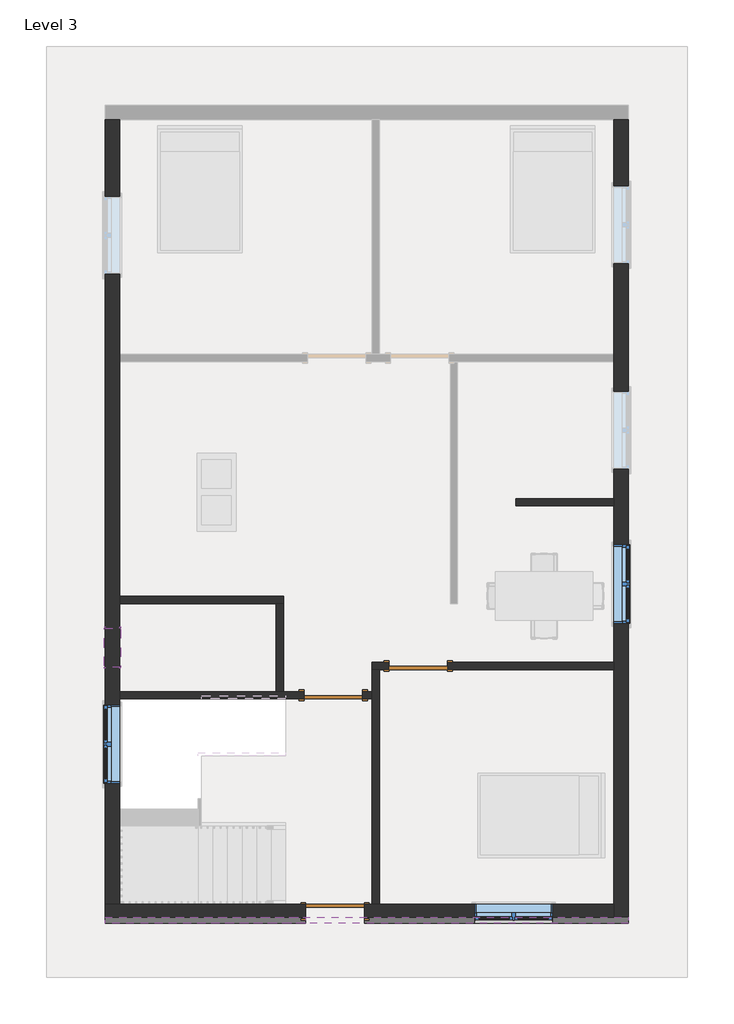
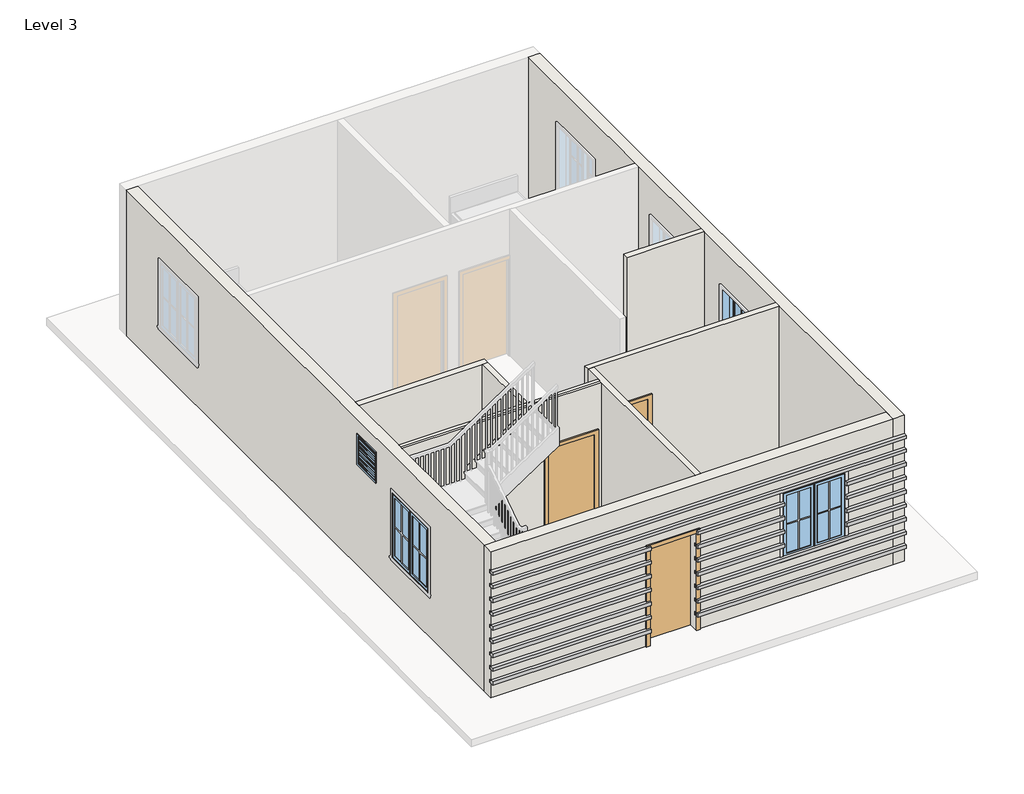
# One storey, part 1 of 3: 9 proxies, 9 walls, 4 windows, 3 doors.
"""IFC4 building model written with IfcOpenShell, lengths in millimetres."""

from ifc_helpers import new_model, si_unit, frame, origin, place, context, project, spatial, polyline, outline, extrude, faceted_brep, transform, mapped, element, save
from components import single_flush_door_3_17d80c48, single_flush_door_3_5e62189b, single_flush_door_3_89fc3733, window_casement_double_window_4_576b2d2c, window_f2d8fef0

model = new_model("IFC4")

# Units and contexts
model_context = context("Model", 3, world=origin())
ifc_project = project(units=[si_unit("LENGTHUNIT", "METRE", prefix="MILLI")], contexts=[model_context])

# Site, building, storey
site = spatial("IfcSite", under=ifc_project)
building = spatial("IfcBuilding", under=site)
storey = spatial("IfcBuildingStorey", under=building, Name="Level 3", Elevation=6248.4)

# Proxies
placement = place(None, origin())
element("IfcBuildingElementProxy", 1, Name="Reveal", ObjectType="Reveal", at=placement, inside=storey, context=model_context, shape_type="SweptSolid", body=[
    extrude(outline(polyline([(2831.4882597, -6585.4426559), (2831.4882597, -6677.5176559), (-1289.6617403, -6677.5176559), (-1289.6617403, -6585.4426559), (2831.4882597, -6585.4426559)])), frame((0.0, 0.0, 6553.2), z_axis=(0.0, 0.0, 1.0), x_axis=(1.0, 0.0, 0.0)), (0.0, 0.0, 1.0), 67.7333333),
    extrude(outline(polyline([(-2204.0617403, -6585.4426559), (-2204.0617403, -6677.5176559), (-5334.6117403, -6677.5176559), (-5334.6117403, -6585.4426559), (-2204.0617403, -6585.4426559)])), frame((0.0, 0.0, 6553.2), z_axis=(0.0, 0.0, 1.0), x_axis=(1.0, 0.0, 0.0)), (0.0, 0.0, 1.0), 67.7333333),
])
element("IfcBuildingElementProxy", 2, Name="Reveal", ObjectType="Reveal", at=placement, inside=storey, context=model_context, shape_type="SweptSolid", body=[
    extrude(outline(polyline([(2831.4882597, -6585.4426559), (2831.4882597, -6677.5176559), (-1289.6617403, -6677.5176559), (-1289.6617403, -6585.4426559), (2831.4882597, -6585.4426559)])), frame((0.0, 0.0, 6839.6994231), z_axis=(0.0, 0.0, 1.0), x_axis=(1.0, 0.0, 0.0)), (0.0, 0.0, 1.0), 67.7333333),
    extrude(outline(polyline([(-2204.0617403, -6585.4426559), (-2204.0617403, -6677.5176559), (-5334.6117403, -6677.5176559), (-5334.6117403, -6585.4426559), (-2204.0617403, -6585.4426559)])), frame((0.0, 0.0, 6839.6994231), z_axis=(0.0, 0.0, 1.0), x_axis=(1.0, 0.0, 0.0)), (0.0, 0.0, 1.0), 67.7333333),
])
element("IfcBuildingElementProxy", 3, Name="Reveal", ObjectType="Reveal", at=placement, inside=storey, context=model_context, shape_type="SweptSolid", body=[
    extrude(outline(polyline([(2831.4882597, -6585.4426559), (2831.4882597, -6677.5176559), (-1289.6617403, -6677.5176559), (-1289.6617403, -6585.4426559), (2831.4882597, -6585.4426559)])), frame((0.0, 0.0, 7126.1988461), z_axis=(0.0, 0.0, 1.0), x_axis=(1.0, 0.0, 0.0)), (0.0, 0.0, 1.0), 67.7333333),
    extrude(outline(polyline([(-2204.0617403, -6585.4426559), (-2204.0617403, -6677.5176559), (-5334.6117403, -6677.5176559), (-5334.6117403, -6585.4426559), (-2204.0617403, -6585.4426559)])), frame((0.0, 0.0, 7126.1988461), z_axis=(0.0, 0.0, 1.0), x_axis=(1.0, 0.0, 0.0)), (0.0, 0.0, 1.0), 67.7333333),
])
element("IfcBuildingElementProxy", 4, Name="Reveal", ObjectType="Reveal", at=placement, inside=storey, context=model_context, shape_type="SweptSolid", body=[
    extrude(outline(polyline([(2831.4882597, -6585.4426559), (2831.4882597, -6677.5176559), (1650.3882597, -6677.5176559), (1650.3882597, -6585.4426559), (2831.4882597, -6585.4426559)])), frame((0.0, 0.0, 7412.6982692), z_axis=(0.0, 0.0, 1.0), x_axis=(1.0, 0.0, 0.0)), (0.0, 0.0, 1.0), 67.7333333),
    extrude(outline(polyline([(431.1882597, -6585.4426559), (431.1882597, -6677.5176559), (-1289.6617403, -6677.5176559), (-1289.6617403, -6585.4426559), (431.1882597, -6585.4426559)])), frame((0.0, 0.0, 7412.6982692), z_axis=(0.0, 0.0, 1.0), x_axis=(1.0, 0.0, 0.0)), (0.0, 0.0, 1.0), 67.7333333),
    extrude(outline(polyline([(-2204.0617403, -6585.4426559), (-2204.0617403, -6677.5176559), (-5334.6117403, -6677.5176559), (-5334.6117403, -6585.4426559), (-2204.0617403, -6585.4426559)])), frame((0.0, 0.0, 7412.6982692), z_axis=(0.0, 0.0, 1.0), x_axis=(1.0, 0.0, 0.0)), (0.0, 0.0, 1.0), 67.7333333),
])
element("IfcBuildingElementProxy", 5, Name="Reveal", ObjectType="Reveal", at=placement, inside=storey, context=model_context, shape_type="SweptSolid", body=[
    extrude(outline(polyline([(2831.4882597, -6585.4426559), (2831.4882597, -6677.5176559), (1650.3882597, -6677.5176559), (1650.3882597, -6585.4426559), (2831.4882597, -6585.4426559)])), frame((0.0, 0.0, 7699.1976923), z_axis=(0.0, 0.0, 1.0), x_axis=(1.0, 0.0, 0.0)), (0.0, 0.0, 1.0), 67.7333333),
    extrude(outline(polyline([(431.1882597, -6585.4426559), (431.1882597, -6677.5176559), (-1289.6617403, -6677.5176559), (-1289.6617403, -6585.4426559), (431.1882597, -6585.4426559)])), frame((0.0, 0.0, 7699.1976923), z_axis=(0.0, 0.0, 1.0), x_axis=(1.0, 0.0, 0.0)), (0.0, 0.0, 1.0), 67.7333333),
    extrude(outline(polyline([(-2204.0617403, -6585.4426559), (-2204.0617403, -6677.5176559), (-5334.6117403, -6677.5176559), (-5334.6117403, -6585.4426559), (-2204.0617403, -6585.4426559)])), frame((0.0, 0.0, 7699.1976923), z_axis=(0.0, 0.0, 1.0), x_axis=(1.0, 0.0, 0.0)), (0.0, 0.0, 1.0), 67.7333333),
])
element("IfcBuildingElementProxy", 6, Name="Reveal", ObjectType="Reveal", at=placement, inside=storey, context=model_context, shape_type="SweptSolid", body=[
    extrude(outline(polyline([(2831.4882597, -6585.4426559), (2831.4882597, -6677.5176559), (1650.3882597, -6677.5176559), (1650.3882597, -6585.4426559), (2831.4882597, -6585.4426559)])), frame((0.0, 0.0, 7985.6971154), z_axis=(0.0, 0.0, 1.0), x_axis=(1.0, 0.0, 0.0)), (0.0, 0.0, 1.0), 67.7333333),
    extrude(outline(polyline([(431.1882597, -6585.4426559), (431.1882597, -6677.5176559), (-1289.6617403, -6677.5176559), (-1289.6617403, -6585.4426559), (431.1882597, -6585.4426559)])), frame((0.0, 0.0, 7985.6971154), z_axis=(0.0, 0.0, 1.0), x_axis=(1.0, 0.0, 0.0)), (0.0, 0.0, 1.0), 67.7333333),
    extrude(outline(polyline([(-2204.0617403, -6585.4426559), (-2204.0617403, -6677.5176559), (-5334.6117403, -6677.5176559), (-5334.6117403, -6585.4426559), (-2204.0617403, -6585.4426559)])), frame((0.0, 0.0, 7985.6971154), z_axis=(0.0, 0.0, 1.0), x_axis=(1.0, 0.0, 0.0)), (0.0, 0.0, 1.0), 67.7333333),
])
element("IfcBuildingElementProxy", 7, Name="Reveal", ObjectType="Reveal", at=placement, inside=storey, context=model_context, shape_type="SweptSolid", body=[
    extrude(outline(polyline([(2831.4882597, -6585.4426559), (2831.4882597, -6677.5176559), (1650.3882597, -6677.5176559), (1650.3882597, -6585.4426559), (2831.4882597, -6585.4426559)])), frame((0.0, 0.0, 8272.1965384), z_axis=(0.0, 0.0, 1.0), x_axis=(1.0, 0.0, 0.0)), (0.0, 0.0, 1.0), 67.7333333),
    extrude(outline(polyline([(431.1882597, -6585.4426559), (431.1882597, -6677.5176559), (-1289.6617403, -6677.5176559), (-1289.6617403, -6585.4426559), (431.1882597, -6585.4426559)])), frame((0.0, 0.0, 8272.1965384), z_axis=(0.0, 0.0, 1.0), x_axis=(1.0, 0.0, 0.0)), (0.0, 0.0, 1.0), 67.7333333),
    extrude(outline(polyline([(-2204.0617403, -6585.4426559), (-2204.0617403, -6677.5176559), (-5334.6117403, -6677.5176559), (-5334.6117403, -6585.4426559), (-2204.0617403, -6585.4426559)])), frame((0.0, 0.0, 8272.1965384), z_axis=(0.0, 0.0, 1.0), x_axis=(1.0, 0.0, 0.0)), (0.0, 0.0, 1.0), 67.7333333),
])
element("IfcBuildingElementProxy", 8, Name="Reveal", ObjectType="Reveal", at=placement, inside=storey, context=model_context, shape_type="SweptSolid", body=[
    extrude(outline(polyline([(2831.4882597, -6585.4426559), (2831.4882597, -6677.5176559), (-5334.6117403, -6677.5176559), (-5334.6117403, -6585.4426559), (2831.4882597, -6585.4426559)])), frame((0.0, 0.0, 8558.6959615), z_axis=(0.0, 0.0, 1.0), x_axis=(1.0, 0.0, 0.0)), (0.0, 0.0, 1.0), 67.7333333),
])
element("IfcBuildingElementProxy", 9, Name="Reveal", ObjectType="Reveal", at=placement, inside=storey, context=model_context, shape_type="SweptSolid", body=[
    extrude(outline(polyline([(2831.4882597, -6585.4426559), (2831.4882597, -6677.5176559), (-5334.6117403, -6677.5176559), (-5334.6117403, -6585.4426559), (2831.4882597, -6585.4426559)])), frame((0.0, 0.0, 8845.1953846), z_axis=(0.0, 0.0, 1.0), x_axis=(1.0, 0.0, 0.0)), (0.0, 0.0, 1.0), 67.7333333),
])

# Doors
single_flush_door_3_shape = single_flush_door_3_17d80c48(model_context)
element("IfcDoor", 10, ObjectType="Single-Flush : DOOR 3'", at=placement, inside=storey, context=model_context, shape_type="MappedRepresentation", body=[
    mapped(single_flush_door_3_shape, transform((-451.4617403, -2667.4926559, 6248.4), x_axis=(-1.0, 0.0, 0.0), y_axis=(0.0, -1.0, 0.0), z_axis=(0.0, 0.0, 1.0))),
])
single_flush_door_3_2_shape = single_flush_door_3_5e62189b(model_context)
element("IfcDoor", 11, ObjectType="Single-Flush : DOOR 3'", at=placement, inside=storey, context=model_context, shape_type="MappedRepresentation", body=[
    mapped(single_flush_door_3_2_shape, transform((-1772.2617403, -3124.6926559, 6248.4), x_axis=(1.0, 0.0, 0.0), y_axis=(0.0, 1.0, 0.0), z_axis=(0.0, 0.0, 1.0))),
])
single_flush_door_3_3_shape = single_flush_door_3_89fc3733(model_context)
element("IfcDoor", 12, ObjectType="Single-Flush : DOOR 3'", at=placement, inside=storey, context=model_context, shape_type="MappedRepresentation", body=[
    mapped(single_flush_door_3_3_shape, transform((-1746.8617403, -6496.5426559, 6248.4), x_axis=(1.0, 0.0, 0.0), y_axis=(0.0, 1.0, 0.0), z_axis=(0.0, 0.0, 1.0))),
])

# Walls
element("IfcWall", 13, ObjectType="ALL 4.5\"", at=placement, inside=storey, context=model_context, shape_type="SweptSolid", body=[
    extrude(outline(polyline([(1078.8882597, -57.6426559), (2602.8882597, -57.6426559), (2602.8882597, -171.9426559), (1078.8882597, -171.9426559), (1078.8882597, -57.6426559)])), frame((0.0, 0.0, 6248.4), z_axis=(0.0, 0.0, 1.0), x_axis=(1.0, 0.0, 0.0)), (0.0, 0.0, 1.0), 3048.0),
])
element("IfcWall", 14, ObjectType="ALL 4.5\"", at=placement, inside=storey, context=model_context, shape_type="Brep", body=[
    faceted_brep([(-908.6617403, -2610.3426559, 8280.4), (-908.6617403, -2610.3426559, 6248.4), (-1169.0117403, -2610.3426559, 6248.4), (-1169.0117403, -2610.3426559, 9296.4), (2602.8882597, -2610.3426559, 9296.4), (2602.8882597, -2610.3426559, 6248.4), (5.7382597, -2610.3426559, 6248.4), (5.7382597, -2610.3426559, 8280.4), (-1169.0117403, -2724.6426559, 6248.4), (-1054.7117403, -2724.6426559, 6248.4), (-908.6617403, -2724.6426559, 6248.4), (-908.6617403, -2724.6426559, 8280.4), (5.7382597, -2724.6426559, 8280.4), (5.7382597, -2724.6426559, 6248.4), (2602.8882597, -2724.6426559, 6248.4), (2602.8882597, -2724.6426559, 9296.4), (-1054.7117403, -2724.6426559, 9296.4), (-1169.0117403, -2724.6426559, 9296.4)], [[[0, 1, 2, 3, 4, 5, 6, 7]], [[8, 9, 10, 11, 12, 13, 14, 15, 16, 17]], [[6, 5, 14, 13]], [[2, 1, 10, 9, 8]], [[5, 4, 15, 14]], [[3, 2, 8, 17]], [[11, 10, 1, 0]], [[12, 11, 0, 7]], [[13, 12, 7, 6]], [[4, 3, 17, 16, 15]]]),
])
element("IfcWall", 15, ObjectType="ALL 4.5\"", at=placement, inside=storey, context=model_context, shape_type="Brep", body=[
    faceted_brep([(-1169.0117403, -2724.6426559, 6248.4), (-1169.0117403, -3067.5426559, 6248.4), (-1169.0117403, -3181.8426559, 6248.4), (-1169.0117403, -6382.2426559, 6248.4), (-1169.0117403, -6382.2426559, 9296.4), (-1169.0117403, -3181.8426559, 9296.4), (-1169.0117403, -3067.5426559, 9296.4), (-1169.0117403, -2724.6426559, 9296.4), (-1054.7117403, -2724.6426559, 6248.4), (-1054.7117403, -2724.6426559, 9296.4), (-1054.7117403, -6382.2426559, 9296.4), (-1054.7117403, -6382.2426559, 6248.4)], [[[0, 1, 2, 3, 4, 5, 6, 7]], [[8, 9, 10, 11]], [[3, 2, 1, 0, 8, 11]], [[0, 7, 9, 8]], [[4, 3, 11, 10]], [[7, 6, 5, 4, 10, 9]]]),
])
element("IfcWall", 16, ObjectType="ALL 4.5\"", at=placement, inside=storey, context=model_context, shape_type="Brep", body=[
    faceted_brep([(-1169.0117403, -3067.5426559, 6248.4), (-1315.0617403, -3067.5426559, 6248.4), (-1315.0617403, -3067.5426559, 8280.4), (-2229.4617403, -3067.5426559, 8280.4), (-2229.4617403, -3067.5426559, 6248.4), (-2553.3117403, -3067.5426559, 6248.4), (-2667.6117403, -3067.5426559, 6248.4), (-5106.0117403, -3067.5426559, 6248.4), (-5106.0117403, -3067.5426559, 9296.4), (-2667.6117403, -3067.5426559, 9296.4), (-2553.3117403, -3067.5426559, 9296.4), (-1169.0117403, -3067.5426559, 9296.4), (-1315.0617403, -3181.8426559, 8280.4), (-1315.0617403, -3181.8426559, 6248.4), (-1169.0117403, -3181.8426559, 6248.4), (-1169.0117403, -3181.8426559, 9296.4), (-5106.0117403, -3181.8426559, 9296.4), (-5106.0117403, -3181.8426559, 6248.4), (-2229.4617403, -3181.8426559, 6248.4), (-2229.4617403, -3181.8426559, 8280.4), (-5106.0117403, -3131.0426559, 9296.4), (-1169.0117403, -3131.0426559, 9296.4), (-2515.2117403, -3131.0426559, 9296.4)], [[[0, 1, 2, 3, 4, 5, 6, 7, 8, 9, 10, 11]], [[12, 13, 14, 15, 16, 17, 18, 19]], [[18, 17, 7, 6, 5, 4]], [[14, 13, 1, 0]], [[8, 7, 17, 16, 20]], [[0, 11, 21, 15, 14]], [[2, 1, 13, 12]], [[3, 2, 12, 19]], [[4, 3, 19, 18]], [[11, 10, 9, 8, 20, 22, 21]], [[20, 16, 15, 21, 22]]]),
])
element("IfcWall", 17, ObjectType="ALL 4.5\"", at=placement, inside=storey, context=model_context, shape_type="Brep", body=[
    faceted_brep([(-5106.0117403, -1695.9426559, 6248.4), (-2667.6117403, -1695.9426559, 6248.4), (-2553.3117403, -1695.9426559, 6248.4), (-2553.3117403, -1695.9426559, 9296.4), (-2667.6117403, -1695.9426559, 9296.4), (-5106.0117403, -1695.9426559, 9296.4), (-5106.0117403, -1581.6426559, 6248.4), (-5106.0117403, -1581.6426559, 9296.4), (-2553.3117403, -1581.6426559, 9296.4), (-2553.3117403, -1581.6426559, 6248.4)], [[[0, 1, 2, 3, 4, 5]], [[6, 7, 8, 9]], [[2, 1, 0, 6, 9]], [[0, 5, 7, 6]], [[3, 2, 9, 8]], [[5, 4, 3, 8, 7]]]),
])
element("IfcWall", 18, ObjectType="ALL 4.5\"", at=placement, inside=storey, context=model_context, shape_type="SweptSolid", body=[
    extrude(outline(polyline([(-2667.6117403, -3067.5426559), (-2667.6117403, -1695.9426559), (-2553.3117403, -1695.9426559), (-2553.3117403, -3067.5426559), (-2667.6117403, -3067.5426559)])), frame((0.0, 0.0, 6248.4), z_axis=(0.0, 0.0, 1.0), x_axis=(1.0, 0.0, 0.0)), (0.0, 0.0, 1.0), 3048.0),
])
element("IfcWall", 19, ObjectType="WALL 9\"", at=placement, inside=storey, context=model_context, shape_type="Brep", body=[
    faceted_brep([(2602.8882597, 5847.8573441, 6248.4), (2602.8882597, 2190.2573441, 6248.4), (2602.8882597, 2075.9573441, 6248.4), (2602.8882597, -57.6426559, 6248.4), (2602.8882597, -171.9426559, 6248.4), (2602.8882597, -2610.3426559, 6248.4), (2602.8882597, -2724.6426559, 6248.4), (2602.8882597, -6382.2426559, 6248.4), (2602.8882597, -6610.8426559, 6248.4), (2602.8882597, -6610.8426559, 6553.2), (2602.8882597, -6585.4426559, 6553.2), (2602.8882597, -6585.4426559, 6620.9333333), (2602.8882597, -6610.8426559, 6620.9333333), (2602.8882597, -6610.8426559, 6839.6994231), (2602.8882597, -6585.4426559, 6839.6994231), (2602.8882597, -6585.4426559, 6907.4327564), (2602.8882597, -6610.8426559, 6907.4327564), (2602.8882597, -6610.8426559, 7126.1988461), (2602.8882597, -6585.4426559, 7126.1988461), (2602.8882597, -6585.4426559, 7193.9321795), (2602.8882597, -6610.8426559, 7193.9321795), (2602.8882597, -6610.8426559, 7412.6982692), (2602.8882597, -6585.4426559, 7412.6982692), (2602.8882597, -6585.4426559, 7480.4316025), (2602.8882597, -6610.8426559, 7480.4316025), (2602.8882597, -6610.8426559, 7699.1976923), (2602.8882597, -6585.4426559, 7699.1976923), (2602.8882597, -6585.4426559, 7766.9310256), (2602.8882597, -6610.8426559, 7766.9310256), (2602.8882597, -6610.8426559, 7985.6971154), (2602.8882597, -6585.4426559, 7985.6971154), (2602.8882597, -6585.4426559, 8053.4304487), (2602.8882597, -6610.8426559, 8053.4304487), (2602.8882597, -6610.8426559, 8272.1965384), (2602.8882597, -6585.4426559, 8272.1965384), (2602.8882597, -6585.4426559, 8339.9298718), (2602.8882597, -6610.8426559, 8339.9298718), (2602.8882597, -6610.8426559, 8558.6959615), (2602.8882597, -6585.4426559, 8558.6959615), (2602.8882597, -6585.4426559, 8626.4292948), (2602.8882597, -6610.8426559, 8626.4292948), (2602.8882597, -6610.8426559, 8845.1953846), (2602.8882597, -6585.4426559, 8845.1953846), (2602.8882597, -6585.4426559, 8912.9287179), (2602.8882597, -6610.8426559, 8912.9287179), (2602.8882597, -6610.8426559, 9296.4), (2602.8882597, -6382.2426559, 9296.4), (2602.8882597, -2724.6426559, 9296.4), (2602.8882597, -2610.3426559, 9296.4), (2602.8882597, -171.9426559, 9296.4), (2602.8882597, -57.6426559, 9296.4), (2602.8882597, 2075.9573441, 9296.4), (2602.8882597, 2190.2573441, 9296.4), (2602.8882597, 5847.8573441, 9296.4), (2602.8882597, 3599.9573441, 8509.0), (2602.8882597, 3599.9573441, 7162.8), (2602.8882597, 4819.1573441, 7162.8), (2602.8882597, 4819.1573441, 8509.0), (2602.8882597, 399.5573441, 8509.0), (2602.8882597, 399.5573441, 7162.8), (2602.8882597, 1618.7573441, 7162.8), (2602.8882597, 1618.7573441, 8509.0), (2602.8882597, -2000.7426559, 8509.0), (2602.8882597, -2000.7426559, 7162.8), (2602.8882597, -781.5426559, 7162.8), (2602.8882597, -781.5426559, 8509.0), (2831.4882597, -6610.8426559, 6248.4), (2831.4882597, 5847.8573441, 6248.4), (2831.4882597, 5847.8573441, 9296.4), (2831.4882597, -6610.8426559, 9296.4), (2831.4882597, -6610.8426559, 8912.9287179), (2831.4882597, -6585.4426559, 8912.9287179), (2831.4882597, -6585.4426559, 8845.1953846), (2831.4882597, -6610.8426559, 8845.1953846), (2831.4882597, -6610.8426559, 8626.4292948), (2831.4882597, -6585.4426559, 8626.4292948), (2831.4882597, -6585.4426559, 8558.6959615), (2831.4882597, -6610.8426559, 8558.6959615), (2831.4882597, -6610.8426559, 8339.9298718), (2831.4882597, -6585.4426559, 8339.9298718), (2831.4882597, -6585.4426559, 8272.1965384), (2831.4882597, -6610.8426559, 8272.1965384), (2831.4882597, -6610.8426559, 8053.4304487), (2831.4882597, -6585.4426559, 8053.4304487), (2831.4882597, -6585.4426559, 7985.6971154), (2831.4882597, -6610.8426559, 7985.6971154), (2831.4882597, -6610.8426559, 7766.9310256), (2831.4882597, -6585.4426559, 7766.9310256), (2831.4882597, -6585.4426559, 7699.1976923), (2831.4882597, -6610.8426559, 7699.1976923), (2831.4882597, -6610.8426559, 7480.4316025), (2831.4882597, -6585.4426559, 7480.4316025), (2831.4882597, -6585.4426559, 7412.6982692), (2831.4882597, -6610.8426559, 7412.6982692), (2831.4882597, -6610.8426559, 7193.9321795), (2831.4882597, -6585.4426559, 7193.9321795), (2831.4882597, -6585.4426559, 7126.1988461), (2831.4882597, -6610.8426559, 7126.1988461), (2831.4882597, -6610.8426559, 6907.4327564), (2831.4882597, -6585.4426559, 6907.4327564), (2831.4882597, -6585.4426559, 6839.6994231), (2831.4882597, -6610.8426559, 6839.6994231), (2831.4882597, -6610.8426559, 6620.9333333), (2831.4882597, -6585.4426559, 6620.9333333), (2831.4882597, -6585.4426559, 6553.2), (2831.4882597, -6610.8426559, 6553.2), (2831.4882597, 3599.9573441, 7162.8), (2831.4882597, 3599.9573441, 8509.0), (2831.4882597, 4819.1573441, 8509.0), (2831.4882597, 4819.1573441, 7162.8), (2831.4882597, 399.5573441, 7162.8), (2831.4882597, 399.5573441, 8509.0), (2831.4882597, 1618.7573441, 8509.0), (2831.4882597, 1618.7573441, 7162.8), (2831.4882597, -2000.7426559, 7162.8), (2831.4882597, -2000.7426559, 8509.0), (2831.4882597, -781.5426559, 8509.0), (2831.4882597, -781.5426559, 7162.8)], [[[0, 1, 2, 3, 4, 5, 6, 7, 8, 9, 10, 11, 12, 13, 14, 15, 16, 17, 18, 19, 20, 21, 22, 23, 24, 25, 26, 27, 28, 29, 30, 31, 32, 33, 34, 35, 36, 37, 38, 39, 40, 41, 42, 43, 44, 45, 46, 47, 48, 49, 50, 51, 52, 53], [54, 55, 56, 57], [58, 59, 60, 61], [62, 63, 64, 65]], [[66, 67, 68, 69, 70, 71, 72, 73, 74, 75, 76, 77, 78, 79, 80, 81, 82, 83, 84, 85, 86, 87, 88, 89, 90, 91, 92, 93, 94, 95, 96, 97, 98, 99, 100, 101, 102, 103, 104, 105], [106, 107, 108, 109], [110, 111, 112, 113], [114, 115, 116, 117]], [[8, 7, 6, 5, 4, 3, 2, 1, 0, 67, 66]], [[0, 53, 68, 67]], [[8, 66, 105, 9]], [[69, 45, 44, 70]], [[12, 102, 101, 13]], [[16, 98, 97, 17]], [[20, 94, 93, 21]], [[24, 90, 89, 25]], [[28, 86, 85, 29]], [[32, 82, 81, 33]], [[36, 78, 77, 37]], [[40, 74, 73, 41]], [[55, 54, 107, 106]], [[56, 55, 106, 109]], [[57, 56, 109, 108]], [[54, 57, 108, 107]], [[59, 58, 111, 110]], [[60, 59, 110, 113]], [[61, 60, 113, 112]], [[58, 61, 112, 111]], [[63, 62, 115, 114]], [[64, 63, 114, 117]], [[65, 64, 117, 116]], [[62, 65, 116, 115]], [[53, 52, 51, 50, 49, 48, 47, 46, 45, 69, 68]], [[11, 103, 102, 12]], [[104, 10, 9, 105]], [[103, 11, 10, 104]], [[15, 99, 98, 16]], [[100, 14, 13, 101]], [[99, 15, 14, 100]], [[19, 95, 94, 20]], [[96, 18, 17, 97]], [[95, 19, 18, 96]], [[23, 91, 90, 24]], [[92, 22, 21, 93]], [[91, 23, 22, 92]], [[27, 87, 86, 28]], [[88, 26, 25, 89]], [[87, 27, 26, 88]], [[31, 83, 82, 32]], [[84, 30, 29, 85]], [[83, 31, 30, 84]], [[35, 79, 78, 36]], [[80, 34, 33, 81]], [[79, 35, 34, 80]], [[39, 75, 74, 40]], [[76, 38, 37, 77]], [[75, 39, 38, 76]], [[43, 71, 70, 44]], [[72, 42, 41, 73]], [[71, 43, 42, 72]]]),
])
element("IfcWall", 20, ObjectType="WALL 9\"", at=placement, inside=storey, context=model_context, shape_type="Brep", body=[
    faceted_brep([(-5334.6117403, -6382.2426559, 9296.4), (-5106.0117403, -6382.2426559, 9296.4), (-1169.0117403, -6382.2426559, 9296.4), (-1054.7117403, -6382.2426559, 9296.4), (2602.8882597, -6382.2426559, 9296.4), (2602.8882597, -6382.2426559, 6248.4), (-1054.7117403, -6382.2426559, 6248.4), (-1169.0117403, -6382.2426559, 6248.4), (-1289.6617403, -6382.2426559, 6248.4), (-1289.6617403, -6382.2426559, 8280.4), (-2204.0617403, -6382.2426559, 8280.4), (-2204.0617403, -6382.2426559, 6248.4), (-5106.0117403, -6382.2426559, 6248.4), (-5334.6117403, -6382.2426559, 6248.4), (431.1882597, -6382.2426559, 8509.0), (431.1882597, -6382.2426559, 7162.8), (1650.3882597, -6382.2426559, 7162.8), (1650.3882597, -6382.2426559, 8509.0), (2602.8882597, -6610.8426559, 9296.4), (-5334.6117403, -6610.8426559, 9296.4), (-5334.6117403, -6610.8426559, 8912.9287179), (2602.8882597, -6610.8426559, 8912.9287179), (431.1882597, -6610.8426559, 8509.0), (1650.3882597, -6610.8426559, 8509.0), (1650.3882597, -6610.8426559, 8339.9298718), (2602.8882597, -6610.8426559, 8339.9298718), (2602.8882597, -6610.8426559, 8558.6959615), (-5334.6117403, -6610.8426559, 8558.6959615), (-5334.6117403, -6610.8426559, 8339.9298718), (-2204.0617403, -6610.8426559, 8339.9298718), (-2204.0617403, -6610.8426559, 8280.4), (-1289.6617403, -6610.8426559, 8280.4), (-1289.6617403, -6610.8426559, 8339.9298718), (431.1882597, -6610.8426559, 8339.9298718), (-5334.6117403, -6610.8426559, 6248.4), (-2204.0617403, -6610.8426559, 6248.4), (-2204.0617403, -6610.8426559, 6553.2), (-5334.6117403, -6610.8426559, 6553.2), (-1289.6617403, -6610.8426559, 6248.4), (2602.8882597, -6610.8426559, 6248.4), (2602.8882597, -6610.8426559, 6553.2), (-1289.6617403, -6610.8426559, 6553.2), (-1289.6617403, -6610.8426559, 6620.9333333), (2602.8882597, -6610.8426559, 6620.9333333), (2602.8882597, -6610.8426559, 6839.6994231), (-1289.6617403, -6610.8426559, 6839.6994231), (-5334.6117403, -6610.8426559, 6620.9333333), (-2204.0617403, -6610.8426559, 6620.9333333), (-2204.0617403, -6610.8426559, 6839.6994231), (-5334.6117403, -6610.8426559, 6839.6994231), (-1289.6617403, -6610.8426559, 6907.4327564), (2602.8882597, -6610.8426559, 6907.4327564), (2602.8882597, -6610.8426559, 7126.1988461), (-1289.6617403, -6610.8426559, 7126.1988461), (-5334.6117403, -6610.8426559, 6907.4327564), (-2204.0617403, -6610.8426559, 6907.4327564), (-2204.0617403, -6610.8426559, 7126.1988461), (-5334.6117403, -6610.8426559, 7126.1988461), (-1289.6617403, -6610.8426559, 7193.9321795), (431.1882597, -6610.8426559, 7193.9321795), (431.1882597, -6610.8426559, 7412.6982692), (-1289.6617403, -6610.8426559, 7412.6982692), (1650.3882597, -6610.8426559, 7193.9321795), (2602.8882597, -6610.8426559, 7193.9321795), (2602.8882597, -6610.8426559, 7412.6982692), (1650.3882597, -6610.8426559, 7412.6982692), (-5334.6117403, -6610.8426559, 7193.9321795), (-2204.0617403, -6610.8426559, 7193.9321795), (-2204.0617403, -6610.8426559, 7412.6982692), (-5334.6117403, -6610.8426559, 7412.6982692), (1650.3882597, -6610.8426559, 7480.4316025), (2602.8882597, -6610.8426559, 7480.4316025), (2602.8882597, -6610.8426559, 7699.1976923), (1650.3882597, -6610.8426559, 7699.1976923), (-1289.6617403, -6610.8426559, 7480.4316025), (431.1882597, -6610.8426559, 7480.4316025), (431.1882597, -6610.8426559, 7699.1976923), (-1289.6617403, -6610.8426559, 7699.1976923), (-5334.6117403, -6610.8426559, 7480.4316025), (-2204.0617403, -6610.8426559, 7480.4316025), (-2204.0617403, -6610.8426559, 7699.1976923), (-5334.6117403, -6610.8426559, 7699.1976923), (1650.3882597, -6610.8426559, 7766.9310256), (2602.8882597, -6610.8426559, 7766.9310256), (2602.8882597, -6610.8426559, 7985.6971154), (1650.3882597, -6610.8426559, 7985.6971154), (-1289.6617403, -6610.8426559, 7766.9310256), (431.1882597, -6610.8426559, 7766.9310256), (431.1882597, -6610.8426559, 7985.6971154), (-1289.6617403, -6610.8426559, 7985.6971154), (-5334.6117403, -6610.8426559, 7766.9310256), (-2204.0617403, -6610.8426559, 7766.9310256), (-2204.0617403, -6610.8426559, 7985.6971154), (-5334.6117403, -6610.8426559, 7985.6971154), (1650.3882597, -6610.8426559, 8053.4304487), (2602.8882597, -6610.8426559, 8053.4304487), (2602.8882597, -6610.8426559, 8272.1965384), (1650.3882597, -6610.8426559, 8272.1965384), (-1289.6617403, -6610.8426559, 8053.4304487), (431.1882597, -6610.8426559, 8053.4304487), (431.1882597, -6610.8426559, 8272.1965384), (-1289.6617403, -6610.8426559, 8272.1965384), (-5334.6117403, -6610.8426559, 8053.4304487), (-2204.0617403, -6610.8426559, 8053.4304487), (-2204.0617403, -6610.8426559, 8272.1965384), (-5334.6117403, -6610.8426559, 8272.1965384), (-5334.6117403, -6610.8426559, 8626.4292948), (2602.8882597, -6610.8426559, 8626.4292948), (2602.8882597, -6610.8426559, 8845.1953846), (-5334.6117403, -6610.8426559, 8845.1953846), (2602.8882597, -6585.4426559, 8912.9287179), (2602.8882597, -6585.4426559, 8845.1953846), (2602.8882597, -6585.4426559, 8626.4292948), (2602.8882597, -6585.4426559, 8558.6959615), (2602.8882597, -6585.4426559, 8339.9298718), (2602.8882597, -6585.4426559, 8272.1965384), (2602.8882597, -6585.4426559, 8053.4304487), (2602.8882597, -6585.4426559, 7985.6971154), (2602.8882597, -6585.4426559, 7766.9310256), (2602.8882597, -6585.4426559, 7699.1976923), (2602.8882597, -6585.4426559, 7480.4316025), (2602.8882597, -6585.4426559, 7412.6982692), (2602.8882597, -6585.4426559, 7193.9321795), (2602.8882597, -6585.4426559, 7126.1988461), (2602.8882597, -6585.4426559, 6907.4327564), (2602.8882597, -6585.4426559, 6839.6994231), (2602.8882597, -6585.4426559, 6620.9333333), (2602.8882597, -6585.4426559, 6553.2), (-5334.6117403, -6585.4426559, 6553.2), (-5334.6117403, -6585.4426559, 6620.9333333), (-5334.6117403, -6585.4426559, 6839.6994231), (-5334.6117403, -6585.4426559, 6907.4327564), (-5334.6117403, -6585.4426559, 7126.1988461), (-5334.6117403, -6585.4426559, 7193.9321795), (-5334.6117403, -6585.4426559, 7412.6982692), (-5334.6117403, -6585.4426559, 7480.4316025), (-5334.6117403, -6585.4426559, 7699.1976923), (-5334.6117403, -6585.4426559, 7766.9310256), (-5334.6117403, -6585.4426559, 7985.6971154), (-5334.6117403, -6585.4426559, 8053.4304487), (-5334.6117403, -6585.4426559, 8272.1965384), (-5334.6117403, -6585.4426559, 8339.9298718), (-5334.6117403, -6585.4426559, 8558.6959615), (-5334.6117403, -6585.4426559, 8626.4292948), (-5334.6117403, -6585.4426559, 8845.1953846), (-5334.6117403, -6585.4426559, 8912.9287179), (431.1882597, -6585.4426559, 8339.9298718), (431.1882597, -6585.4426559, 8272.1965384), (431.1882597, -6585.4426559, 8053.4304487), (431.1882597, -6585.4426559, 7985.6971154), (431.1882597, -6585.4426559, 7766.9310256), (431.1882597, -6585.4426559, 7699.1976923), (431.1882597, -6585.4426559, 7480.4316025), (431.1882597, -6585.4426559, 7412.6982692), (431.1882597, -6585.4426559, 7193.9321795), (431.1882597, -6585.4426559, 7162.8), (1650.3882597, -6585.4426559, 7162.8), (1650.3882597, -6585.4426559, 7193.9321795), (1650.3882597, -6585.4426559, 7412.6982692), (1650.3882597, -6585.4426559, 7480.4316025), (1650.3882597, -6585.4426559, 7699.1976923), (1650.3882597, -6585.4426559, 7766.9310256), (1650.3882597, -6585.4426559, 7985.6971154), (1650.3882597, -6585.4426559, 8053.4304487), (1650.3882597, -6585.4426559, 8272.1965384), (1650.3882597, -6585.4426559, 8339.9298718), (-1289.6617403, -6585.4426559, 6553.2), (-1289.6617403, -6585.4426559, 6620.9333333), (-1289.6617403, -6585.4426559, 6839.6994231), (-1289.6617403, -6585.4426559, 6907.4327564), (-1289.6617403, -6585.4426559, 7126.1988461), (-1289.6617403, -6585.4426559, 7193.9321795), (-1289.6617403, -6585.4426559, 7412.6982692), (-1289.6617403, -6585.4426559, 7480.4316025), (-1289.6617403, -6585.4426559, 7699.1976923), (-1289.6617403, -6585.4426559, 7766.9310256), (-1289.6617403, -6585.4426559, 7985.6971154), (-1289.6617403, -6585.4426559, 8053.4304487), (-1289.6617403, -6585.4426559, 8272.1965384), (-1289.6617403, -6585.4426559, 8280.4), (-2204.0617403, -6585.4426559, 8280.4), (-2204.0617403, -6585.4426559, 8272.1965384), (-2204.0617403, -6585.4426559, 8053.4304487), (-2204.0617403, -6585.4426559, 7985.6971154), (-2204.0617403, -6585.4426559, 7766.9310256), (-2204.0617403, -6585.4426559, 7699.1976923), (-2204.0617403, -6585.4426559, 7480.4316025), (-2204.0617403, -6585.4426559, 7412.6982692), (-2204.0617403, -6585.4426559, 7193.9321795), (-2204.0617403, -6585.4426559, 7126.1988461), (-2204.0617403, -6585.4426559, 6907.4327564), (-2204.0617403, -6585.4426559, 6839.6994231), (-2204.0617403, -6585.4426559, 6620.9333333), (-2204.0617403, -6585.4426559, 6553.2), (-1289.6617403, -6585.4426559, 8339.9298718), (-2204.0617403, -6585.4426559, 8339.9298718)], [[[0, 1, 2, 3, 4, 5, 6, 7, 8, 9, 10, 11, 12, 13], [14, 15, 16, 17]], [[18, 19, 20, 21]], [[22, 23, 24, 25, 26, 27, 28, 29, 30, 31, 32, 33]], [[34, 35, 36, 37]], [[38, 39, 40, 41]], [[42, 43, 44, 45]], [[46, 47, 48, 49]], [[50, 51, 52, 53]], [[54, 55, 56, 57]], [[58, 59, 60, 61]], [[62, 63, 64, 65]], [[66, 67, 68, 69]], [[70, 71, 72, 73]], [[74, 75, 76, 77]], [[78, 79, 80, 81]], [[82, 83, 84, 85]], [[86, 87, 88, 89]], [[90, 91, 92, 93]], [[94, 95, 96, 97]], [[98, 99, 100, 101]], [[102, 103, 104, 105]], [[106, 107, 108, 109]], [[5, 39, 38, 8, 7, 6]], [[34, 13, 12, 11, 35]], [[4, 3, 2, 1, 0, 19, 18]], [[5, 4, 18, 21, 110, 111, 108, 107, 112, 113, 26, 25, 114, 115, 96, 95, 116, 117, 84, 83, 118, 119, 72, 71, 120, 121, 64, 63, 122, 123, 52, 51, 124, 125, 44, 43, 126, 127, 40, 39]], [[0, 13, 34, 37, 128, 129, 46, 49, 130, 131, 54, 57, 132, 133, 66, 69, 134, 135, 78, 81, 136, 137, 90, 93, 138, 139, 102, 105, 140, 141, 28, 27, 142, 143, 106, 109, 144, 145, 20, 19]], [[15, 14, 22, 33, 146, 147, 100, 99, 148, 149, 88, 87, 150, 151, 76, 75, 152, 153, 60, 59, 154, 155]], [[16, 15, 155, 156]], [[17, 16, 156, 157, 62, 65, 158, 159, 70, 73, 160, 161, 82, 85, 162, 163, 94, 97, 164, 165, 24, 23]], [[14, 17, 23, 22]], [[9, 8, 38, 41, 166, 167, 42, 45, 168, 169, 50, 53, 170, 171, 58, 61, 172, 173, 74, 77, 174, 175, 86, 89, 176, 177, 98, 101, 178, 179]], [[10, 9, 179, 31, 30, 180]], [[11, 10, 180, 181, 104, 103, 182, 183, 92, 91, 184, 185, 80, 79, 186, 187, 68, 67, 188, 189, 56, 55, 190, 191, 48, 47, 192, 193, 36, 35]], [[167, 126, 43, 42]], [[127, 166, 41, 40]], [[126, 167, 166, 127]], [[129, 192, 47, 46]], [[193, 128, 37, 36]], [[192, 129, 128, 193]], [[169, 124, 51, 50]], [[125, 168, 45, 44]], [[124, 169, 168, 125]], [[131, 190, 55, 54]], [[191, 130, 49, 48]], [[190, 131, 130, 191]], [[171, 154, 59, 58]], [[157, 122, 63, 62]], [[123, 170, 53, 52]], [[154, 171, 170, 123, 122, 157, 156, 155]], [[133, 188, 67, 66]], [[189, 132, 57, 56]], [[188, 133, 132, 189]], [[159, 120, 71, 70]], [[121, 158, 65, 64]], [[120, 159, 158, 121]], [[173, 152, 75, 74]], [[153, 172, 61, 60]], [[152, 173, 172, 153]], [[135, 186, 79, 78]], [[187, 134, 69, 68]], [[186, 135, 134, 187]], [[161, 118, 83, 82]], [[119, 160, 73, 72]], [[118, 161, 160, 119]], [[175, 150, 87, 86]], [[151, 174, 77, 76]], [[150, 175, 174, 151]], [[137, 184, 91, 90]], [[185, 136, 81, 80]], [[184, 137, 136, 185]], [[163, 116, 95, 94]], [[117, 162, 85, 84]], [[116, 163, 162, 117]], [[177, 148, 99, 98]], [[149, 176, 89, 88]], [[148, 177, 176, 149]], [[139, 182, 103, 102]], [[183, 138, 93, 92]], [[182, 139, 138, 183]], [[165, 114, 25, 24]], [[115, 164, 97, 96]], [[114, 165, 164, 115]], [[179, 194, 32, 31]], [[194, 146, 33, 32]], [[147, 178, 101, 100]], [[146, 194, 179, 178, 147]], [[195, 180, 30, 29]], [[141, 195, 29, 28]], [[181, 140, 105, 104]], [[195, 141, 140, 181, 180]], [[143, 112, 107, 106]], [[113, 142, 27, 26]], [[112, 143, 142, 113]], [[145, 110, 21, 20]], [[111, 144, 109, 108]], [[110, 145, 144, 111]]]),
])
element("IfcWall", 21, ObjectType="WALL 9\"", at=placement, inside=storey, context=model_context, shape_type="Brep", body=[
    faceted_brep([(-5106.0117403, -6382.2426559, 6248.4), (-5106.0117403, -3181.8426559, 6248.4), (-5106.0117403, -3067.5426559, 6248.4), (-5106.0117403, -1695.9426559, 6248.4), (-5106.0117403, -1581.6426559, 6248.4), (-5106.0117403, 2075.9573441, 6248.4), (-5106.0117403, 2190.2573441, 6248.4), (-5106.0117403, 5847.8573441, 6248.4), (-5106.0117403, 5847.8573441, 9296.4), (-5106.0117403, 2190.2573441, 9296.4), (-5106.0117403, 2075.9573441, 9296.4), (-5106.0117403, -1581.6426559, 9296.4), (-5106.0117403, -1695.9426559, 9296.4), (-5106.0117403, -3067.5426559, 9296.4), (-5106.0117403, -3181.8426559, 9296.4), (-5106.0117403, -6382.2426559, 9296.4), (-5106.0117403, -3277.0926559, 8509.0), (-5106.0117403, -3277.0926559, 7162.8), (-5106.0117403, -4496.2926559, 7162.8), (-5106.0117403, -4496.2926559, 8509.0), (-5106.0117403, 4657.2323441, 8509.0), (-5106.0117403, 4657.2323441, 7162.8), (-5106.0117403, 3438.0323441, 7162.8), (-5106.0117403, 3438.0323441, 8509.0), (-5106.0117403, -2686.5426559, 8991.6), (-5106.0117403, -2076.9426559, 8991.6), (-5106.0117403, -2076.9426559, 8382.0), (-5106.0117403, -2686.5426559, 8382.0), (-5334.6117403, -6382.2426559, 6248.4), (-5334.6117403, -6382.2426559, 9296.4), (-5334.6117403, 5847.8573441, 9296.4), (-5334.6117403, 5847.8573441, 6248.4), (-5334.6117403, -3277.0926559, 8509.0), (-5334.6117403, -4496.2926559, 8509.0), (-5334.6117403, -4496.2926559, 7162.8), (-5334.6117403, -3277.0926559, 7162.8), (-5334.6117403, 4657.2323441, 8509.0), (-5334.6117403, 3438.0323441, 8509.0), (-5334.6117403, 3438.0323441, 7162.8), (-5334.6117403, 4657.2323441, 7162.8), (-5334.6117403, -2686.5426559, 8991.6), (-5334.6117403, -2686.5426559, 8382.0), (-5334.6117403, -2076.9426559, 8382.0), (-5334.6117403, -2076.9426559, 8991.6)], [[[0, 1, 2, 3, 4, 5, 6, 7, 8, 9, 10, 11, 12, 13, 14, 15], [16, 17, 18, 19], [20, 21, 22, 23], [24, 25, 26, 27]], [[28, 29, 30, 31], [32, 33, 34, 35], [36, 37, 38, 39], [40, 41, 42, 43]], [[7, 6, 5, 4, 3, 2, 1, 0, 28, 31]], [[15, 14, 13, 12, 11, 10, 9, 8, 30, 29]], [[8, 7, 31, 30]], [[0, 15, 29, 28]], [[17, 16, 32, 35]], [[18, 17, 35, 34]], [[19, 18, 34, 33]], [[16, 19, 33, 32]], [[21, 20, 36, 39]], [[22, 21, 39, 38]], [[23, 22, 38, 37]], [[20, 23, 37, 36]], [[41, 40, 24, 27]], [[42, 41, 27, 26]], [[43, 42, 26, 25]], [[40, 43, 25, 24]]]),
])

# Windows
window_casement_double_window_4_shape = window_casement_double_window_4_576b2d2c(model_context)
element("IfcWindow", 22, ObjectType="Window-Casement-Double : WINDOW 4'", at=placement, inside=storey, context=model_context, shape_type="MappedRepresentation", body=[
    mapped(window_casement_double_window_4_shape, transform((-5220.3117403, -3886.6926559, 6248.4), x_axis=(0.0, 1.0, 0.0), y_axis=(-1.0, 0.0, 0.0), z_axis=(0.0, 0.0, 1.0))),
])
element("IfcWindow", 23, ObjectType="Window-Casement-Double : WINDOW 4'", at=placement, inside=storey, context=model_context, shape_type="MappedRepresentation", body=[
    mapped(window_casement_double_window_4_shape, transform((2717.1882597, -1391.1426559, 6248.4), x_axis=(0.0, -1.0, 0.0), y_axis=(1.0, 0.0, 0.0), z_axis=(0.0, 0.0, 1.0))),
])
element("IfcWindow", 24, ObjectType="Window-Casement-Double : WINDOW 4'", at=placement, inside=storey, context=model_context, shape_type="MappedRepresentation", body=[
    mapped(window_casement_double_window_4_shape, transform((1040.7882597, -6496.5426559, 6248.4), x_axis=(-1.0, 0.0, 0.0), y_axis=(0.0, -1.0, 0.0), z_axis=(0.0, 0.0, 1.0))),
])
window_shape = window_f2d8fef0(model_context)
element("IfcWindow", 25, ObjectType="Window-Louvers : 24\" x 24\"", at=placement, inside=storey, context=model_context, shape_type="MappedRepresentation", body=[
    mapped(window_shape, transform((-5226.6617403, -2381.7426559, 7467.6), x_axis=(0.0, 1.0, 0.0), y_axis=(-1.0, 0.0, 0.0), z_axis=(0.0, 0.0, 1.0))),
])

save(model, "model.ifc")

# Revit data of these elements
# Type "Single-Flush : DOOR 3'"
#   Type Mark = "8"
#   Construction Type Id = "MDOOR"
#   Assembly Code = "C1020"
#   Analytic Construction = "Metal"
#   Thickness = 0' - 2"
#   Heat Transfer Coefficient (U) = 0.651978 BTU/(h·ft²·°F)
#   Height = 6' - 8"
#   Trim Projection Ext = 0' - 1"
#   Trim Projection Int = 0' - 1"
#   Trim Width = 0' - 3"
#   Width = 3' - 0"
#   Define Thermal Properties by = 1
#   Door Material = Door - Panel
#   Frame Material = Door - Frame
#   Visual Light Transmittance = 0
#   Solar Heat Gain Coefficient = 0
#   Function = (empty or 0)
#   Wall Closure = (empty or 0)
# Type "ALL 4.5\""
#   Assembly Code = "B2010"
#   Layers, outside or top first: 0' - 4 1/2" no material (function 1)
# Type "WALL 9\""
#   Assembly Code = "B2010"
#   Layers, outside or top first: 0' - 9" "Carpet (1)" (function 1)
# Type "Window-Casement-Double : WINDOW 4'"
#   Type Mark = "18"
#   Fire Rating = "0.5h"
#   Assembly Code = "B2020100"
#   Analytic Construction = "Double glazing - domestic"
#   Frame Extension [instance default] = 0' - 0 1/4"
#   Window Inset [instance default] = 0' - 0"
#   Wall Thickness [instance default] = 0' - 6"
#   Interior Wall Closure [instance default] = 0' - 2 1/4"
#   Half Width = 2' - 0"
#   Visual Light Transmittance = 0.81
#   Thermal Resistance (R) = 1.8146 (h·ft²·°F)/BTU
#   Solar Heat Gain Coefficient = 0.76
#   Rough Width = 4' - 0 1/2"
#   Rough Height = 4' - 5 1/2"
#   Height = 4' - 5"
#   Heat Transfer Coefficient (U) = 0.5511 BTU/(h·ft²·°F)
#   Exterior Wall Closure [instance default] = 0' - 1 1/4"
#   Extension Jamb [instance default] = 0' - 2 1/4"
#   Default Sill Height = 3' - 0"
#   Width = 4' - 0"
#   Muntin Visibility = yes
#   Interior Trim Visibility [instance default] = yes
#   Exterior Trim Visibility [instance default] = yes
#   Extension Jamb Visibility [instance default] = yes
#   Interior Trim Material = Wood - Stained
#   Muntin Pattern = Muntin Pattern_2x2 : Muntin Pattern_2x2
#   Interior Trim = Trim-Window-Interior-Flat : Picture Frame
#   Interior Frame Material = Wood - Stained
#   Glass Panel Material = Glass
#   Exterior Trim Material = Clad - White
#   Exterior Trim = Trim-Window-Exterior-Flat : with Sill
#   Exterior Frame Material = Clad - White
#   Wall Closure = (empty or 0)
# Type "Window-Louvers : 24\" x 24\""
#   Type Mark = "19"
#   Construction Type Id = "GSP4R"
#   Assembly Code = "B20"
#   Analytic Construction = "1/8 in Pilkington single glazing"
#   Visual Light Transmittance = 0.9
#   Thermal Resistance (R) = 1.53941 (h·ft²·°F)/BTU
#   Solar Heat Gain Coefficient = 0.78
#   Max Height = 1' - 11.74264"
#   Height = 2' - 0"
#   Heat Transfer Coefficient (U) = 0.6496 BTU/(h·ft²·°F)
#   Blade Width [instance default] = 1' - 10 1/2"
#   Blade Vertical Thickness = 0' - 0.35355"
#   Blade Thickness = 0' - 0 1/4"
#   Blade Spacing = 0' - 1 1/2"
#   Blade Height = 0' - 1.85355"
#   Blade Depth = 0' - 3"
#   Blade Angle = 45.00°
#   Default Sill Height = 3' - 0"
#   Trim Projection_Exterior = 0' - 0 1/2"
#   Trim Projection_Interior = 0' - 0 1/2"
#   Trim Width_Exterior = 0' - 1 1/2"
#   Trim Width_Interior = 0' - 1 1/2"
#   Width = 2' - 0"
#   Max Blade Count = 12
#   Define Thermal Properties by = 1
#   Blade Count = 12
#   Frame Material = Birch
#   Louver Material = Birch
#   Trim Exterior Material = Birch
#   Trim Interior Material = Birch
#   Wall Closure = (empty or 0)
# Elements 10, 11, 12 (IfcDoor, "Single-Flush : DOOR 3'")
#   Phase Created = New Construction
#   Materials on its faces: "Door - Frame", "Door - Panel"
# Elements 13, 17, 18 (IfcWall, "ALL 4.5\"")
#   Top Offset = 0' - 0"
#   Base Offset = 0' - 0"
#   Unconnected Height = 10' - 0"
#   wall height = 10' - 0"
#   Phase Created = New Construction
#   Base Constraint = Level 3
#   Materials on its faces: "Default Wall"
# Elements 14, 15, 16 (IfcWall, "ALL 4.5\"")
#   Top Offset = 0' - 0"
#   Base Offset = 0' - 0"
#   Unconnected Height = 10' - 0"
#   wall height = 10' - 0"
#   Phase Created = New Construction
#   Base Constraint = Level 3
#   Materials on its faces: "Default Wall", "Clad - White"
# Element 19 (IfcWall, "WALL 9\"")
#   Top Offset = 0' - 0"
#   Base Offset = 0' - 0"
#   Unconnected Height = 10' - 0"
#   wall height = 10' - 0"
#   Phase Created = New Construction
#   Base Constraint = Level 3
#   Materials on its faces: "Carpet (1)", "Wood - Stained"
# Elements 20, 21 (IfcWall, "WALL 9\"")
#   Top Offset = 0' - 0"
#   Base Offset = 0' - 0"
#   Unconnected Height = 10' - 0"
#   wall height = 10' - 0"
#   Phase Created = New Construction
#   Base Constraint = Level 3
#   Materials on its faces: "Carpet (1)", "Clad - White", "Wood - Stained"
# Element 22 (IfcWindow, "Window-Casement-Double : WINDOW 4'")
#   Mark = "15"
#   Window Inset = 0' - 0"
#   Interior Wall Closure = 0' - 2 1/4"
#   Frame Extension = 0' - 0 1/4"
#   Exterior Wall Closure = 0' - 1 1/4"
#   Interior Trim Visibility = yes
#   Exterior Trim Visibility = yes
#   Phase Created = New Construction
#   Materials on its faces: "Wood - Stained", "Glass", "Clad - White"
# Element 23 (IfcWindow, "Window-Casement-Double : WINDOW 4'")
#   Mark = "19"
#   Window Inset = 0' - 0"
#   Interior Wall Closure = 0' - 2 1/4"
#   Frame Extension = 0' - 0 1/4"
#   Exterior Wall Closure = 0' - 1 1/4"
#   Interior Trim Visibility = yes
#   Exterior Trim Visibility = yes
#   Phase Created = New Construction
#   Materials on its faces: "Wood - Stained", "Glass", "Clad - White"
# Element 24 (IfcWindow, "Window-Casement-Double : WINDOW 4'")
#   Mark = "20"
#   Window Inset = 0' - 0"
#   Interior Wall Closure = 0' - 2 1/4"
#   Frame Extension = 0' - 0 1/4"
#   Exterior Wall Closure = 0' - 1 1/4"
#   Interior Trim Visibility = yes
#   Exterior Trim Visibility = yes
#   Phase Created = New Construction
#   Materials on its faces: "Wood - Stained", "Glass", "Clad - White"
# Element 25 (IfcWindow, "Window-Louvers : 24\" x 24\"")
#   Mark = "21"
#   Blade Width = 1' - 10 1/2"
#   Phase Created = New Construction
#   Materials on its faces: "Birch"
# Materials
#   "Door - Panel": class "Wood", colour RGB 210 159 95, transparency 0, Cost = 0
#   "Door - Frame": colour RGB 118 70 51, transparency 0, Cost = 0
#   "Carpet (1)": class "Carpet", colour RGB 124 80 67, transparency 0, Description = "Interior finish", Cost = 0
#   "Wood - Stained": class "Wood", colour RGB 224 178 126, transparency 0, Cost = 0
#   "Glass": class "Glass", colour RGB 0 128 192, transparency 0.75, Description = "Soda Lime Glass", Cost = 0
#   "Clad - White": class "Wood", colour RGB 242 242 238, transparency 0, Cost = 0
#   "Birch": class "Wood", colour RGB 224 178 126, transparency 0, Description = "Betula Alleghaniensis", Cost = 0
#   "Default Wall": colour RGB 128 128 128, transparency 0, Cost = 0
